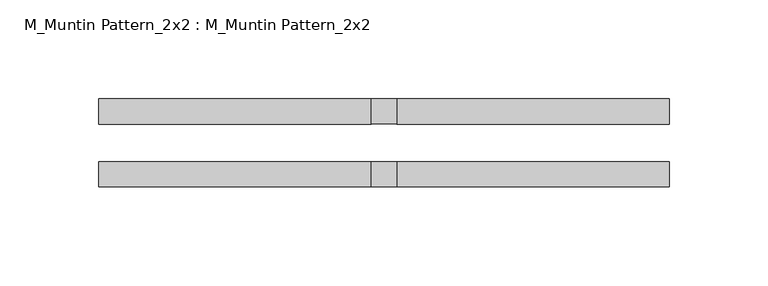
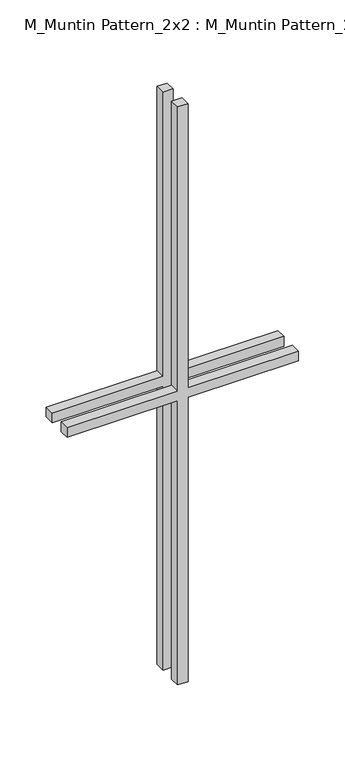
"""IFC4 building model written with IfcOpenShell, lengths in millimetres: proxy geometry, M_Muntin Pattern_2x2 : M_Muntin Pattern_2x2."""

from ifc_helpers import new_model, si_unit, frame, origin, place, context, project, spatial, polyline, outline, extrude, source, transform, mapped, element, save


def m_muntin_pattern_2x2_m_muntin_pattern_2x2_62480ac4(model_context):
    return source(origin(), model_context, "Body", "SweptSolid", [
        extrude(outline(polyline([(386.5, -6.35), (386.5, -144.2375), (373.8, -144.2375), (373.8, -6.35), (0.0, -6.35), (0.0, 6.35), (373.8, 6.35), (373.8, 144.2375), (386.5, 144.2375), (386.5, 6.35), (760.3, 6.35), (760.3, -6.35), (386.5, -6.35)])), frame((0.0, 9.525, 0.0), z_axis=(0.0, 1.0, 0.0), x_axis=(0.0, 0.0, 1.0)), (0.0, 0.0, 1.0), 12.7),
        extrude(outline(polyline([(386.5, -6.35), (386.5, -144.2375), (373.8, -144.2375), (373.8, -6.35), (0.0, -6.35), (0.0, 6.35), (373.8, 6.35), (373.8, 144.2375), (386.5, 144.2375), (386.5, 6.35), (760.3, 6.35), (760.3, -6.35), (386.5, -6.35)])), frame((0.0, -22.225, 0.0), z_axis=(0.0, 1.0, 0.0), x_axis=(0.0, 0.0, 1.0)), (0.0, 0.0, 1.0), 12.7),
    ])


if __name__ == "__main__":
    model = new_model("IFC4")
    model_context = context("Model", 3, world=origin())
    ifc_project = project(units=[si_unit("LENGTHUNIT", "METRE", prefix="MILLI")], contexts=[model_context])
    site = spatial("IfcSite", under=ifc_project)
    building = spatial("IfcBuilding", under=site)
    placement = place(None, origin())
    m_muntin_pattern_2x2_m_muntin_pattern_2x2_shape = m_muntin_pattern_2x2_m_muntin_pattern_2x2_62480ac4(model_context)
    element("IfcBuildingElementProxy", 1, Name="M_Muntin Pattern_2x2 : M_Muntin Pattern_2x2", ObjectType="M_Muntin Pattern_2x2 : M_Muntin Pattern_2x2", at=placement, inside=building, context=model_context, shape_type="MappedRepresentation", body=[
        mapped(m_muntin_pattern_2x2_m_muntin_pattern_2x2_shape, transform((0.0, 0.0, 0.0), x_axis=(1.0, 0.0, 0.0), y_axis=(0.0, 1.0, 0.0), z_axis=(0.0, 0.0, 1.0))),
    ])
    save(model, "model.ifc")

# Revit data of these elements
# Type "M_Muntin Pattern_2x2 : M_Muntin Pattern_2x2"
#   Width [instance default] = 3.937008 ft
#   Thickness = 0.041667 ft
#   Height [instance default] = 3.937008 ft
#   Distance = 0.0625 ft
#   Interior Material [instance default] = none
#   Exterior Material [instance default] = none
#   Default Elevation = 0
# Element 1 (IfcBuildingElementProxy, "M_Muntin Pattern_2x2 : M_Muntin Pattern_2x2")
#   Width = 0.94644 ft
#   Height = 2.494423 ft
#   Interior Material = Wood - Stained
#   Exterior Material = Clad - White
#   Materials on its faces: "Clad - White", "Wood - Stained"
# Materials
#   "Clad - White": class "Wood", colour RGB 242 242 238, transparency 0, Cost = 0
#   "Wood - Stained": class "Wood", colour RGB 224 178 126, transparency 0, Cost = 0
